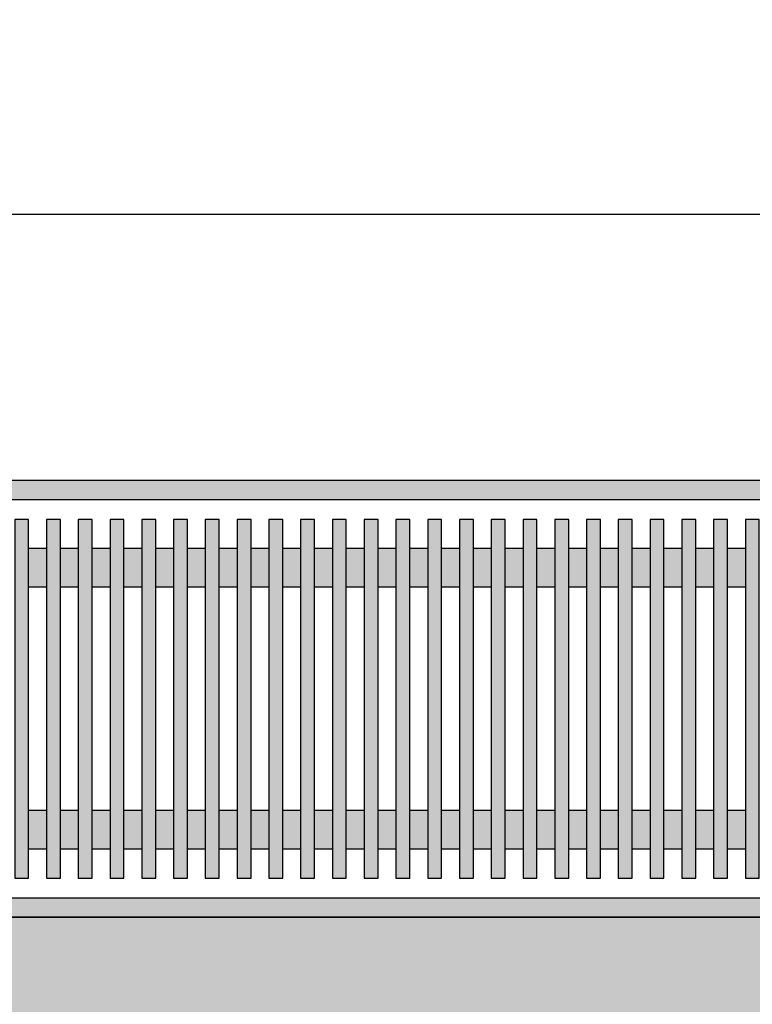
# Model space of a CAD drawing. Units: inches. Extents: x 3592 to 4861, y 1650 to 2243.
# Tile 13 of 30: x 4306 to 4335, y 1772 to 1812. Entities that reach past the tile are written whole.
import ezdxf

# ---------------------------------------------------------------- set-up
doc = ezdxf.new("R2010")
doc.units = ezdxf.units.IN
for name, color, linetype, lineweight in [('A-ANNO-DIMS', 2, 'Continuous', 13), ('A-FURN', 9, 'Continuous', 13), ('A-WALL', 7, 'Continuous', 35), ('estofado', 7, 'Continuous', 25)]:
    doc.layers.add(name, color=color, linetype=linetype, lineweight=lineweight)
doc.layers.add('A-WALL-PATT', color=252, linetype='Continuous', lineweight=13, true_color=0x939598)
doc.layers.add('MOBIL', color=7, linetype='Continuous')
doc.styles.get("Standard").update_dxf_attribs({"font": 'arial.ttf'})
doc.dimstyles.new('ISO-25', dxfattribs={"dimtxt": 9, "dimasz": 2.5, "dimexe": 1.25, "dimexo": 0.625, "dimtad": 1, "dimlunit": 3, "dimtxsty": 'Standard', "dimcen": 2.5, "dimadec": 0, "dimazin": 0, "dimtfac": 1, "dimtmove": 0, "dimatfit": 3, "dimfxl": 1, "dimarcsym": 0})

# ---------------------------------------------------------------- blocks, each defined once
blk = doc.blocks.new('Aparador Aido WV')
at = {"layer": 'MOBIL'}
h = blk.add_hatch(color=256, dxfattribs=at)
h.set_gradient(color1=(226, 228, 228), one_color=1, tint=1, name='CYLINDER')
h.paths.add_polyline_path([(0.9, -0.02), (0.9, 0), (-0.9, 0), (-0.9, -0.02)])
h = blk.add_hatch(color=256, dxfattribs=at)
h.set_gradient(color1=(106, 79, 62), color2=(55, 41, 32), one_color=1, tint=0.17)
h.paths.add_polyline_path([(-0.2072, -0.4098), (-0.1928, -0.4098), (-0.1928, -0.0402), (-0.2072, -0.0402)])
h = blk.add_hatch(color=256, dxfattribs=at)
h.set_gradient(color1=(106, 79, 62), color2=(55, 41, 32), one_color=1, tint=0.17)
h.paths.add_polyline_path([(-0.1744, -0.0402), (-0.1744, -0.4098), (-0.1601, -0.4098), (-0.1601, -0.0402)])
h = blk.add_hatch(color=256, dxfattribs=at)
h.set_gradient(color1=(106, 79, 62), color2=(55, 41, 32), one_color=1, tint=0.17)
h.paths.add_polyline_path([(-0.1417, -0.0402), (-0.1417, -0.4098), (-0.1273, -0.4098), (-0.1273, -0.0402)])
h = blk.add_hatch(color=256, dxfattribs=at)
h.set_gradient(color1=(106, 79, 62), color2=(55, 41, 32), one_color=1, tint=0.17)
h.paths.add_polyline_path([(-0.1089, -0.0402), (-0.1089, -0.4098), (-0.0946, -0.4098), (-0.0946, -0.0402)])
h = blk.add_hatch(color=256, dxfattribs=at)
h.set_gradient(color1=(106, 79, 62), color2=(55, 41, 32), one_color=1, tint=0.17)
h.paths.add_polyline_path([(-0.0762, -0.0402), (-0.0762, -0.4098), (-0.0618, -0.4098), (-0.0618, -0.0402)])
h = blk.add_hatch(color=256, dxfattribs=at)
h.set_gradient(color1=(106, 79, 62), color2=(55, 41, 32), one_color=1, tint=0.17)
h.paths.add_polyline_path([(-0.0434, -0.0402), (-0.0434, -0.4098), (-0.0291, -0.4098), (-0.0291, -0.0402)])
h = blk.add_hatch(color=256, dxfattribs=at)
h.set_gradient(color1=(106, 79, 62), color2=(55, 41, 32), one_color=1, tint=0.17)
h.paths.add_polyline_path([(-0.0107, -0.0402), (-0.0107, -0.4098), (0.0037, -0.4098), (0.0037, -0.0402)])
h = blk.add_hatch(color=256, dxfattribs=at)
h.set_gradient(color1=(106, 79, 62), color2=(55, 41, 32), one_color=1, tint=0.17)
h.paths.add_polyline_path([(0.0221, -0.0402), (0.0221, -0.4098), (0.0364, -0.4098), (0.0364, -0.0402)])
h = blk.add_hatch(color=256, dxfattribs=at)
h.set_gradient(color1=(106, 79, 62), color2=(55, 41, 32), one_color=1, tint=0.17)
h.paths.add_polyline_path([(0.0548, -0.0402), (0.0548, -0.4098), (0.0692, -0.4098), (0.0692, -0.0402)])
h = blk.add_hatch(color=256, dxfattribs=at)
h.set_gradient(color1=(106, 79, 62), color2=(55, 41, 32), one_color=1, tint=0.17)
h.paths.add_polyline_path([(0.1019, -0.0402), (0.0876, -0.0402), (0.0876, -0.4098), (0.1019, -0.4098)])
h = blk.add_hatch(color=256, dxfattribs=at)
h.set_gradient(color1=(106, 79, 62), color2=(55, 41, 32), one_color=1, tint=0.17)
h.paths.add_polyline_path([(0.1203, -0.0402), (0.1203, -0.4098), (0.1347, -0.4098), (0.1347, -0.0402)])
h = blk.add_hatch(color=256, dxfattribs=at)
h.set_gradient(color1=(106, 79, 62), color2=(55, 41, 32), one_color=1, tint=0.17)
h.paths.add_polyline_path([(0.1531, -0.0402), (0.1531, -0.4098), (0.1675, -0.4098), (0.1675, -0.0402)])
h = blk.add_hatch(color=256, dxfattribs=at)
h.set_gradient(color1=(106, 79, 62), color2=(55, 41, 32), one_color=1, tint=0.17)
h.paths.add_polyline_path([(0.1858, -0.0402), (0.1858, -0.4098), (0.2002, -0.4098), (0.2002, -0.0402)])
h = blk.add_hatch(color=256, dxfattribs=at)
h.set_gradient(color1=(106, 79, 62), color2=(55, 41, 32), one_color=1, tint=0.17)
h.paths.add_polyline_path([(0.2186, -0.0402), (0.2186, -0.4098), (0.233, -0.4098), (0.233, -0.0402)])
h = blk.add_hatch(color=256, dxfattribs=at)
h.set_gradient(color1=(106, 79, 62), color2=(55, 41, 32), one_color=1, tint=0.17)
h.paths.add_polyline_path([(0.2513, -0.0402), (0.2513, -0.4098), (0.2657, -0.4098), (0.2657, -0.0402)])
h = blk.add_hatch(color=256, dxfattribs=at)
h.set_gradient(color1=(106, 79, 62), color2=(55, 41, 32), one_color=1, tint=0.17)
h.paths.add_polyline_path([(0.2841, -0.0402), (0.2841, -0.4098), (0.2985, -0.4098), (0.2985, -0.0402)])
h = blk.add_hatch(color=256, dxfattribs=at)
h.set_gradient(color1=(106, 79, 62), color2=(55, 41, 32), one_color=1, tint=0.17)
h.paths.add_polyline_path([(0.3168, -0.0402), (0.3168, -0.4098), (0.3312, -0.4098), (0.3312, -0.0402)])
h = blk.add_hatch(color=256, dxfattribs=at)
h.set_gradient(color1=(106, 79, 62), color2=(55, 41, 32), one_color=1, tint=0.17)
h.paths.add_polyline_path([(0.3496, -0.0402), (0.3496, -0.4098), (0.364, -0.4098), (0.364, -0.0402)])
h = blk.add_hatch(color=256, dxfattribs=at)
h.set_gradient(color1=(106, 79, 62), color2=(55, 41, 32), one_color=1, tint=0.17)
h.paths.add_polyline_path([(0.3823, -0.0402), (0.3823, -0.4098), (0.3967, -0.4098), (0.3967, -0.0402)])
h = blk.add_hatch(color=256, dxfattribs=at)
h.set_gradient(color1=(106, 79, 62), color2=(55, 41, 32), one_color=1, tint=0.17)
h.paths.add_polyline_path([(0.4151, -0.4098), (0.4295, -0.4098), (0.4295, -0.0402), (0.4151, -0.0402)])
h = blk.add_hatch(color=256, dxfattribs=at)
h.set_gradient(color1=(106, 79, 62), color2=(55, 41, 32), one_color=1, tint=0.17)
h.paths.add_polyline_path([(0.4479, -0.0402), (0.4479, -0.4098), (0.4622, -0.4098), (0.4622, -0.0402)])
h = blk.add_hatch(color=256, dxfattribs=at)
h.set_gradient(color1=(106, 79, 62), color2=(55, 41, 32), one_color=1, tint=0.17)
h.paths.add_polyline_path([(0.4806, -0.0402), (0.4806, -0.4098), (0.495, -0.4098), (0.495, -0.0402)])
h = blk.add_hatch(color=256, dxfattribs=at)
h.set_gradient(color1=(106, 79, 62), color2=(55, 41, 32), one_color=1, tint=0.17)
h.paths.add_polyline_path([(0.5134, -0.0402), (0.5134, -0.4098), (0.5277, -0.4098), (0.5277, -0.0402)])
h = blk.add_hatch(color=256, dxfattribs=at)
h.set_gradient(color1=(106, 79, 62), color2=(55, 41, 32), one_color=1, tint=0.17)
h.paths.add_polyline_path([(0.5461, -0.0402), (0.5461, -0.4098), (0.5605, -0.4098), (0.5605, -0.0402)])
h = blk.add_hatch(color=256, dxfattribs=at)
h.set_gradient(color1=(106, 79, 62), color2=(157, 117, 92), one_color=1, tint=0.49)
h.paths.add_polyline_path([(-0.1744, -0.07), (-0.1928, -0.07), (-0.1928, -0.11), (-0.1744, -0.11)])
h = blk.add_hatch(color=256, dxfattribs=at)
h.set_gradient(color1=(106, 79, 62), color2=(157, 117, 92), one_color=1, tint=0.49)
h.paths.add_polyline_path([(-0.1417, -0.07), (-0.1601, -0.07), (-0.1601, -0.11), (-0.1417, -0.11)])
h = blk.add_hatch(color=256, dxfattribs=at)
h.set_gradient(color1=(106, 79, 62), color2=(157, 117, 92), one_color=1, tint=0.49)
h.paths.add_polyline_path([(-0.1089, -0.07), (-0.1273, -0.07), (-0.1273, -0.11), (-0.1089, -0.11)])
h = blk.add_hatch(color=256, dxfattribs=at)
h.set_gradient(color1=(106, 79, 62), color2=(157, 117, 92), one_color=1, tint=0.49)
h.paths.add_polyline_path([(-0.0762, -0.07), (-0.0946, -0.07), (-0.0946, -0.11), (-0.0762, -0.11)])
h = blk.add_hatch(color=256, dxfattribs=at)
h.set_gradient(color1=(106, 79, 62), color2=(157, 117, 92), one_color=1, tint=0.49)
h.paths.add_polyline_path([(-0.0434, -0.07), (-0.0618, -0.07), (-0.0618, -0.11), (-0.0434, -0.11)])
h = blk.add_hatch(color=256, dxfattribs=at)
h.set_gradient(color1=(106, 79, 62), color2=(157, 117, 92), one_color=1, tint=0.49)
h.paths.add_polyline_path([(-0.0107, -0.07), (-0.0291, -0.07), (-0.0291, -0.11), (-0.0107, -0.11)])
h = blk.add_hatch(color=256, dxfattribs=at)
h.set_gradient(color1=(106, 79, 62), color2=(157, 117, 92), one_color=1, tint=0.49)
h.paths.add_polyline_path([(0.0221, -0.07), (0.0037, -0.07), (0.0037, -0.11), (0.0221, -0.11)])
h = blk.add_hatch(color=256, dxfattribs=at)
h.set_gradient(color1=(106, 79, 62), color2=(157, 117, 92), one_color=1, tint=0.49)
h.paths.add_polyline_path([(0.0548, -0.07), (0.0364, -0.07), (0.0364, -0.11), (0.0548, -0.11)])
h = blk.add_hatch(color=256, dxfattribs=at)
h.set_gradient(color1=(106, 79, 62), color2=(157, 117, 92), one_color=1, tint=0.49)
h.paths.add_polyline_path([(0.0876, -0.07), (0.0692, -0.07), (0.0692, -0.11), (0.0876, -0.11)])
h = blk.add_hatch(color=256, dxfattribs=at)
h.set_gradient(color1=(106, 79, 62), color2=(157, 117, 92), one_color=1, tint=0.49)
h.paths.add_polyline_path([(0.1203, -0.07), (0.1019, -0.07), (0.1019, -0.11), (0.1203, -0.11)])
h = blk.add_hatch(color=256, dxfattribs=at)
h.set_gradient(color1=(106, 79, 62), color2=(157, 117, 92), one_color=1, tint=0.49)
h.paths.add_polyline_path([(0.1531, -0.07), (0.1347, -0.07), (0.1347, -0.11), (0.1531, -0.11)])
h = blk.add_hatch(color=256, dxfattribs=at)
h.set_gradient(color1=(106, 79, 62), color2=(157, 117, 92), one_color=1, tint=0.49)
h.paths.add_polyline_path([(0.1858, -0.07), (0.1675, -0.07), (0.1675, -0.11), (0.1858, -0.11)])
h = blk.add_hatch(color=256, dxfattribs=at)
h.set_gradient(color1=(106, 79, 62), color2=(157, 117, 92), one_color=1, tint=0.49)
h.paths.add_polyline_path([(0.2186, -0.07), (0.2002, -0.07), (0.2002, -0.11), (0.2186, -0.11)])
h = blk.add_hatch(color=256, dxfattribs=at)
h.set_gradient(color1=(106, 79, 62), color2=(157, 117, 92), one_color=1, tint=0.49)
h.paths.add_polyline_path([(0.2513, -0.07), (0.233, -0.07), (0.233, -0.11), (0.2513, -0.11)])
h = blk.add_hatch(color=256, dxfattribs=at)
h.set_gradient(color1=(106, 79, 62), color2=(157, 117, 92), one_color=1, tint=0.49)
h.paths.add_polyline_path([(0.2841, -0.07), (0.2657, -0.07), (0.2657, -0.11), (0.2841, -0.11)])
h = blk.add_hatch(color=256, dxfattribs=at)
h.set_gradient(color1=(106, 79, 62), color2=(157, 117, 92), one_color=1, tint=0.49)
h.paths.add_polyline_path([(0.3168, -0.07), (0.2985, -0.07), (0.2985, -0.11), (0.3168, -0.11)])
h = blk.add_hatch(color=256, dxfattribs=at)
h.set_gradient(color1=(106, 79, 62), color2=(157, 117, 92), one_color=1, tint=0.49)
h.paths.add_polyline_path([(0.3496, -0.07), (0.3312, -0.07), (0.3312, -0.11), (0.3496, -0.11)])
h = blk.add_hatch(color=256, dxfattribs=at)
h.set_gradient(color1=(106, 79, 62), color2=(157, 117, 92), one_color=1, tint=0.49)
h.paths.add_polyline_path([(0.3823, -0.07), (0.364, -0.07), (0.364, -0.11), (0.3823, -0.11)])
h = blk.add_hatch(color=256, dxfattribs=at)
h.set_gradient(color1=(106, 79, 62), color2=(157, 117, 92), one_color=1, tint=0.49)
h.paths.add_polyline_path([(0.4151, -0.07), (0.3967, -0.07), (0.3967, -0.11), (0.4151, -0.11)])
h = blk.add_hatch(color=256, dxfattribs=at)
h.set_gradient(color1=(106, 79, 62), color2=(157, 117, 92), one_color=1, tint=0.49)
h.paths.add_polyline_path([(0.4479, -0.07), (0.4295, -0.07), (0.4295, -0.11), (0.4479, -0.11)])
h = blk.add_hatch(color=256, dxfattribs=at)
h.set_gradient(color1=(106, 79, 62), color2=(157, 117, 92), one_color=1, tint=0.49)
h.paths.add_polyline_path([(0.4806, -0.07), (0.4622, -0.07), (0.4622, -0.11), (0.4806, -0.11)])
h = blk.add_hatch(color=256, dxfattribs=at)
h.set_gradient(color1=(106, 79, 62), color2=(157, 117, 92), one_color=1, tint=0.49)
h.paths.add_polyline_path([(0.5134, -0.07), (0.495, -0.07), (0.495, -0.11), (0.5134, -0.11)])
h = blk.add_hatch(color=256, dxfattribs=at)
h.set_gradient(color1=(106, 79, 62), color2=(157, 117, 92), one_color=1, tint=0.49)
h.paths.add_polyline_path([(0.5277, -0.11), (0.5461, -0.11), (0.5461, -0.07), (0.5277, -0.07)])
h = blk.add_hatch(color=256, dxfattribs=at)
h.set_gradient(color1=(106, 79, 62), color2=(157, 117, 92), one_color=1, tint=0.49)
h.paths.add_polyline_path([(-0.1744, -0.34), (-0.1928, -0.34), (-0.1928, -0.38), (-0.1744, -0.38)])
h = blk.add_hatch(color=256, dxfattribs=at)
h.set_gradient(color1=(106, 79, 62), color2=(157, 117, 92), one_color=1, tint=0.49)
h.paths.add_polyline_path([(-0.1417, -0.34), (-0.1601, -0.34), (-0.1601, -0.38), (-0.1417, -0.38)])
h = blk.add_hatch(color=256, dxfattribs=at)
h.set_gradient(color1=(106, 79, 62), color2=(157, 117, 92), one_color=1, tint=0.49)
h.paths.add_polyline_path([(-0.1089, -0.34), (-0.1273, -0.34), (-0.1273, -0.38), (-0.1089, -0.38)])
h = blk.add_hatch(color=256, dxfattribs=at)
h.set_gradient(color1=(106, 79, 62), color2=(157, 117, 92), one_color=1, tint=0.49)
h.paths.add_polyline_path([(-0.0762, -0.34), (-0.0946, -0.34), (-0.0946, -0.38), (-0.0762, -0.38)])
h = blk.add_hatch(color=256, dxfattribs=at)
h.set_gradient(color1=(106, 79, 62), color2=(157, 117, 92), one_color=1, tint=0.49)
h.paths.add_polyline_path([(-0.0434, -0.34), (-0.0618, -0.34), (-0.0618, -0.38), (-0.0434, -0.38)])
h = blk.add_hatch(color=256, dxfattribs=at)
h.set_gradient(color1=(106, 79, 62), color2=(157, 117, 92), one_color=1, tint=0.49)
h.paths.add_polyline_path([(-0.0107, -0.34), (-0.0291, -0.34), (-0.0291, -0.38), (-0.0107, -0.38)])
h = blk.add_hatch(color=256, dxfattribs=at)
h.set_gradient(color1=(106, 79, 62), color2=(157, 117, 92), one_color=1, tint=0.49)
h.paths.add_polyline_path([(0.0221, -0.34), (0.0037, -0.34), (0.0037, -0.38), (0.0221, -0.38)])
h = blk.add_hatch(color=256, dxfattribs=at)
h.set_gradient(color1=(106, 79, 62), color2=(157, 117, 92), one_color=1, tint=0.49)
h.paths.add_polyline_path([(0.0548, -0.34), (0.0364, -0.34), (0.0364, -0.38), (0.0548, -0.38)])
h = blk.add_hatch(color=256, dxfattribs=at)
h.set_gradient(color1=(106, 79, 62), color2=(157, 117, 92), one_color=1, tint=0.49)
h.paths.add_polyline_path([(0.0876, -0.34), (0.0692, -0.34), (0.0692, -0.38), (0.0876, -0.38)])
h = blk.add_hatch(color=256, dxfattribs=at)
h.set_gradient(color1=(106, 79, 62), color2=(157, 117, 92), one_color=1, tint=0.49)
h.paths.add_polyline_path([(0.1203, -0.34), (0.1019, -0.34), (0.1019, -0.38), (0.1203, -0.38)])
h = blk.add_hatch(color=256, dxfattribs=at)
h.set_gradient(color1=(106, 79, 62), color2=(157, 117, 92), one_color=1, tint=0.49)
h.paths.add_polyline_path([(0.1531, -0.34), (0.1347, -0.34), (0.1347, -0.38), (0.1531, -0.38)])
h = blk.add_hatch(color=256, dxfattribs=at)
h.set_gradient(color1=(106, 79, 62), color2=(157, 117, 92), one_color=1, tint=0.49)
h.paths.add_polyline_path([(0.1858, -0.34), (0.1675, -0.34), (0.1675, -0.38), (0.1858, -0.38)])
h = blk.add_hatch(color=256, dxfattribs=at)
h.set_gradient(color1=(106, 79, 62), color2=(157, 117, 92), one_color=1, tint=0.49)
h.paths.add_polyline_path([(0.2186, -0.34), (0.2002, -0.34), (0.2002, -0.38), (0.2186, -0.38)])
h = blk.add_hatch(color=256, dxfattribs=at)
h.set_gradient(color1=(106, 79, 62), color2=(157, 117, 92), one_color=1, tint=0.49)
h.paths.add_polyline_path([(0.2513, -0.34), (0.233, -0.34), (0.233, -0.38), (0.2513, -0.38)])
h = blk.add_hatch(color=256, dxfattribs=at)
h.set_gradient(color1=(106, 79, 62), color2=(157, 117, 92), one_color=1, tint=0.49)
h.paths.add_polyline_path([(0.2841, -0.34), (0.2657, -0.34), (0.2657, -0.38), (0.2841, -0.38)])
h = blk.add_hatch(color=256, dxfattribs=at)
h.set_gradient(color1=(106, 79, 62), color2=(157, 117, 92), one_color=1, tint=0.49)
h.paths.add_polyline_path([(0.3168, -0.34), (0.2985, -0.34), (0.2985, -0.38), (0.3168, -0.38)])
h = blk.add_hatch(color=256, dxfattribs=at)
h.set_gradient(color1=(106, 79, 62), color2=(157, 117, 92), one_color=1, tint=0.49)
h.paths.add_polyline_path([(0.3496, -0.34), (0.3312, -0.34), (0.3312, -0.38), (0.3496, -0.38)])
h = blk.add_hatch(color=256, dxfattribs=at)
h.set_gradient(color1=(106, 79, 62), color2=(157, 117, 92), one_color=1, tint=0.49)
h.paths.add_polyline_path([(0.3823, -0.34), (0.364, -0.34), (0.364, -0.38), (0.3823, -0.38)])
h = blk.add_hatch(color=256, dxfattribs=at)
h.set_gradient(color1=(106, 79, 62), color2=(157, 117, 92), one_color=1, tint=0.49)
h.paths.add_polyline_path([(0.4151, -0.34), (0.3967, -0.34), (0.3967, -0.38), (0.4151, -0.38)])
h = blk.add_hatch(color=256, dxfattribs=at)
h.set_gradient(color1=(106, 79, 62), color2=(157, 117, 92), one_color=1, tint=0.49)
h.paths.add_polyline_path([(0.4479, -0.34), (0.4295, -0.34), (0.4295, -0.38), (0.4479, -0.38)])
h = blk.add_hatch(color=256, dxfattribs=at)
h.set_gradient(color1=(106, 79, 62), color2=(157, 117, 92), one_color=1, tint=0.49)
h.paths.add_polyline_path([(0.4806, -0.34), (0.4622, -0.34), (0.4622, -0.38), (0.4806, -0.38)])
h = blk.add_hatch(color=256, dxfattribs=at)
h.set_gradient(color1=(106, 79, 62), color2=(157, 117, 92), one_color=1, tint=0.49)
h.paths.add_polyline_path([(0.5134, -0.34), (0.495, -0.34), (0.495, -0.38), (0.5134, -0.38)])
h = blk.add_hatch(color=256, dxfattribs=at)
h.set_gradient(color1=(106, 79, 62), color2=(157, 117, 92), one_color=1, tint=0.49)
h.paths.add_polyline_path([(0.5461, -0.34), (0.5277, -0.34), (0.5277, -0.38), (0.5461, -0.38)])
h = blk.add_hatch(color=256, dxfattribs=at)
h.set_gradient(color1=(226, 228, 228), one_color=1, tint=1, name='CYLINDER')
h.paths.add_polyline_path([(0.9, -0.45), (0.9, -0.43), (-0.9, -0.43), (-0.9, -0.45)])
at = {"layer": 'estofado', "ltscale": 0.5}
for p, q in [((-0.1928, -0.07), (-0.1744, -0.07)), ((-0.1601, -0.07), (-0.1417, -0.07)), ((-0.1273, -0.07), (-0.1089, -0.07)), ((-0.0946, -0.07), (-0.0762, -0.07)), ((-0.0618, -0.07), (-0.0434, -0.07)), ((-0.0291, -0.07), (-0.0107, -0.07)), ((0.0037, -0.07), (0.0221, -0.07)), ((0.0364, -0.07), (0.0548, -0.07)), ((0.0692, -0.07), (0.0876, -0.07)), ((0.1019, -0.07), (0.1203, -0.07)), ((0.1347, -0.07), (0.1531, -0.07)), ((0.1675, -0.07), (0.1858, -0.07)), ((0.2002, -0.07), (0.2186, -0.07)), ((0.233, -0.07), (0.2513, -0.07)), ((0.2657, -0.07), (0.2841, -0.07)), ((0.2985, -0.07), (0.3168, -0.07)), ((0.3312, -0.07), (0.3496, -0.07)), ((0.364, -0.07), (0.3823, -0.07)), ((0.3967, -0.07), (0.4151, -0.07)), ((0.4295, -0.07), (0.4479, -0.07)), ((0.4622, -0.07), (0.4806, -0.07)), ((0.495, -0.07), (0.5134, -0.07)), ((0.5277, -0.07), (0.5461, -0.07)), ((-0.1928, -0.11), (-0.1744, -0.11)), ((-0.1601, -0.11), (-0.1417, -0.11)), ((-0.1273, -0.11), (-0.1089, -0.11)), ((-0.0946, -0.11), (-0.0762, -0.11)), ((-0.0618, -0.11), (-0.0434, -0.11)), ((-0.0291, -0.11), (-0.0107, -0.11)), ((0.0037, -0.11), (0.0221, -0.11)), ((0.0364, -0.11), (0.0548, -0.11)), ((0.0692, -0.11), (0.0876, -0.11)), ((0.1019, -0.11), (0.1203, -0.11)), ((0.1347, -0.11), (0.1531, -0.11)), ((0.1675, -0.11), (0.1858, -0.11)), ((0.2002, -0.11), (0.2186, -0.11)), ((0.233, -0.11), (0.2513, -0.11)), ((0.2657, -0.11), (0.2841, -0.11)), ((0.2985, -0.11), (0.3168, -0.11)), ((0.3312, -0.11), (0.3496, -0.11)), ((0.364, -0.11), (0.3823, -0.11)), ((0.3967, -0.11), (0.4151, -0.11)), ((0.4295, -0.11), (0.4479, -0.11)), ((0.4622, -0.11), (0.4806, -0.11)), ((0.495, -0.11), (0.5134, -0.11)), ((0.5277, -0.11), (0.5461, -0.11)), ((-0.1928, -0.34), (-0.1744, -0.34)), ((-0.1601, -0.34), (-0.1417, -0.34)), ((-0.1273, -0.34), (-0.1089, -0.34)), ((-0.0946, -0.34), (-0.0762, -0.34)), ((-0.0618, -0.34), (-0.0434, -0.34)), ((-0.0291, -0.34), (-0.0107, -0.34)), ((0.0037, -0.34), (0.0221, -0.34)), ((0.0364, -0.34), (0.0548, -0.34)), ((0.0692, -0.34), (0.0876, -0.34)), ((0.1019, -0.34), (0.1203, -0.34)), ((0.1347, -0.34), (0.1531, -0.34)), ((0.1675, -0.34), (0.1858, -0.34)), ((0.2002, -0.34), (0.2186, -0.34)), ((0.233, -0.34), (0.2513, -0.34)), ((0.2657, -0.34), (0.2841, -0.34)), ((0.2985, -0.34), (0.3168, -0.34)), ((0.3312, -0.34), (0.3496, -0.34)), ((0.364, -0.34), (0.3823, -0.34)), ((0.3967, -0.34), (0.4151, -0.34)), ((0.4295, -0.34), (0.4479, -0.34)), ((0.4622, -0.34), (0.4806, -0.34)), ((0.495, -0.34), (0.5134, -0.34)), ((0.5277, -0.34), (0.5461, -0.34)), ((-0.1928, -0.38), (-0.1744, -0.38)), ((-0.1601, -0.38), (-0.1417, -0.38)), ((-0.1273, -0.38), (-0.1089, -0.38)), ((-0.0946, -0.38), (-0.0762, -0.38)), ((-0.0618, -0.38), (-0.0434, -0.38)), ((-0.0291, -0.38), (-0.0107, -0.38)), ((0.0037, -0.38), (0.0221, -0.38)), ((0.0364, -0.38), (0.0548, -0.38)), ((0.0692, -0.38), (0.0876, -0.38)), ((0.1019, -0.38), (0.1203, -0.38)), ((0.1347, -0.38), (0.1531, -0.38)), ((0.1675, -0.38), (0.1858, -0.38)), ((0.2002, -0.38), (0.2186, -0.38)), ((0.233, -0.38), (0.2513, -0.38)), ((0.2657, -0.38), (0.2841, -0.38)), ((0.2985, -0.38), (0.3168, -0.38)), ((0.3312, -0.38), (0.3496, -0.38)), ((0.364, -0.38), (0.3823, -0.38)), ((0.3967, -0.38), (0.4151, -0.38)), ((0.4295, -0.38), (0.4479, -0.38)), ((0.4622, -0.38), (0.4806, -0.38)), ((0.495, -0.38), (0.5134, -0.38)), ((0.5277, -0.38), (0.5461, -0.38))]:
    blk.add_line(p, q, dxfattribs=at)
for points in [[(-0.2072, -0.0402), (-0.2072, -0.4098), (-0.1928, -0.4098), (-0.1928, -0.0402)], [(-0.1744, -0.0402), (-0.1744, -0.4098), (-0.1601, -0.4098), (-0.1601, -0.0402)], [(-0.1417, -0.0402), (-0.1417, -0.4098), (-0.1273, -0.4098), (-0.1273, -0.0402)], [(-0.1089, -0.0402), (-0.1089, -0.4098), (-0.0946, -0.4098), (-0.0946, -0.0402)], [(-0.0762, -0.0402), (-0.0762, -0.4098), (-0.0618, -0.4098), (-0.0618, -0.0402)], [(-0.0434, -0.0402), (-0.0434, -0.4098), (-0.0291, -0.4098), (-0.0291, -0.0402)], [(-0.0107, -0.0402), (-0.0107, -0.4098), (0.0037, -0.4098), (0.0037, -0.0402)], [(0.0221, -0.0402), (0.0221, -0.4098), (0.0364, -0.4098), (0.0364, -0.0402)], [(0.0548, -0.0402), (0.0548, -0.4098), (0.0692, -0.4098), (0.0692, -0.0402)], [(0.0876, -0.0402), (0.0876, -0.4098), (0.1019, -0.4098), (0.1019, -0.0402)], [(0.1203, -0.0402), (0.1203, -0.4098), (0.1347, -0.4098), (0.1347, -0.0402)], [(0.1531, -0.0402), (0.1531, -0.4098), (0.1675, -0.4098), (0.1675, -0.0402)], [(0.1858, -0.0402), (0.1858, -0.4098), (0.2002, -0.4098), (0.2002, -0.0402)], [(0.2186, -0.0402), (0.2186, -0.4098), (0.233, -0.4098), (0.233, -0.0402)], [(0.2513, -0.0402), (0.2513, -0.4098), (0.2657, -0.4098), (0.2657, -0.0402)], [(0.2841, -0.0402), (0.2841, -0.4098), (0.2985, -0.4098), (0.2985, -0.0402)], [(0.3168, -0.0402), (0.3168, -0.4098), (0.3312, -0.4098), (0.3312, -0.0402)], [(0.3496, -0.0402), (0.3496, -0.4098), (0.364, -0.4098), (0.364, -0.0402)], [(0.3823, -0.0402), (0.3823, -0.4098), (0.3967, -0.4098), (0.3967, -0.0402)], [(0.4151, -0.0402), (0.4151, -0.4098), (0.4295, -0.4098), (0.4295, -0.0402)], [(0.4479, -0.0402), (0.4479, -0.4098), (0.4622, -0.4098), (0.4622, -0.0402)], [(0.4806, -0.0402), (0.4806, -0.4098), (0.495, -0.4098), (0.495, -0.0402)], [(0.5134, -0.0402), (0.5134, -0.4098), (0.5277, -0.4098), (0.5277, -0.0402)], [(0.5461, -0.0402), (0.5461, -0.4098), (0.5605, -0.4098), (0.5605, -0.0402)]]:
    blk.add_lwpolyline(points, close=True, dxfattribs=at)
at = {"layer": 'MOBIL'}
for p, q in [((0.9, -0.02), (-0.9, -0.02)), ((-0.9, -0.43), (0.9, -0.43))]:
    blk.add_line(p, q, dxfattribs=at)
blk.add_lwpolyline([(-0.9, -0.45), (0.9, -0.45), (0.9, 0), (-0.9, 0)], close=True, dxfattribs=at)
blk = doc.blocks.new('*D156')
at = {"layer": 'A-ANNO-DIMS', "color": 0, "lineweight": -2, "transparency": 16777216}
for p, q in [((4291.393, 1793.561), (4291.393, 1804.979)), ((4363.347, 1793.561), (4363.347, 1804.979)), ((4291.393, 1803.729), (4155.277, 1803.729)), ((4360.847, 1803.729), (4293.893, 1803.729))]:
    blk.add_line(p, q, dxfattribs=at)
at = {"layer": 'A-ANNO-DIMS', "color": 0, "transparency": 16777216}
for points in [[(4293.893, 1804.145), (4293.893, 1803.312), (4291.393, 1803.729)], [(4360.847, 1804.145), (4360.847, 1803.312), (4363.347, 1803.729)]]:
    blk.add_solid(points, dxfattribs=at)
at = {"layer": 'Defpoints', "color": 0, "transparency": 16777216}
for p in [(4291.393, 1803.729), (4291.393, 1792.936), (4363.347, 1792.936)]:
    blk.add_point(p, dxfattribs=at)
at = {"layer": 'A-ANNO-DIMS', "color": 0, "transparency": 16777216, "insert": (4222.085, 1809.01), "char_height": 9, "attachment_point": 5}
blk.add_mtext('SIDEBOARD 6\'-0" TYP.', dxfattribs=at)

msp = doc.modelspace()

# ---------------------------------------------------------------- hatches: boundary and pattern name
at = {"layer": 'A-WALL-PATT'}
h = msp.add_hatch(color=256, dxfattribs=at)
h.dxf.hatch_style = 1
h.paths.add_polyline_path([(4398.37, 2165.219), (4038.37, 2165.219), (4038.37, 1993.219), (4047.37, 1993.219), (4047.37, 2156.219), (4191.37, 2156.219), (4191.37, 2150.219), (4195.37, 2150.219), (4195.37, 2156.219), (4256.37, 2156.219), (4256.37, 2150.219), (4265.37, 2150.219), (4265.37, 2156.219), (4389.37, 2156.219), (4389.37, 2114.219), (4398.37, 2114.219)])
h.paths.add_polyline_path([(4265.37, 2102.219), (4256.37, 2102.219), (4256.37, 2096.219), (4195.37, 2096.219), (4195.37, 2102.219), (4191.37, 2102.219), (4191.37, 2020.219), (4195.37, 2020.219), (4195.37, 2087.219), (4256.37, 2087.219), (4256.37, 2020.219), (4306.37, 2020.219), (4306.37, 2024.219), (4265.37, 2024.219)], flags=17)
h.paths.add_polyline_path([(4398.37, 2066.219), (4389.37, 2066.219), (4389.37, 2024.219), (4348.37, 2024.219), (4348.37, 2020.219), (4389.37, 2020.219), (4389.37, 1989.719), (4398.37, 1989.719)])
h.paths.add_polyline_path([(4398.37, 1941.719), (4389.37, 1941.719), (4389.37, 1911.219), (4301.37, 1911.219), (4301.37, 1907.219), (4389.37, 1907.219), (4389.37, 1865.219), (4398.37, 1865.219)])
h.paths.add_polyline_path([(4398.37, 1817.219), (4389.37, 1817.219), (4389.37, 1775.219), (4265.37, 1775.219), (4265.37, 1911.219), (4256.37, 1911.219), (4256.37, 1817.219), (4220.87, 1817.219), (4220.87, 1808.219), (4256.37, 1808.219), (4256.37, 1766.219), (4389.37, 1766.219), (4389.37, 1694.219), (4256.37, 1694.219), (4256.37, 1685.219), (4398.37, 1685.219)])
h.paths.add_polyline_path([(4178.87, 1817.219), (4077.37, 1817.219), (4077.37, 1808.219), (4178.87, 1808.219)])
h.paths.add_polyline_path([(4111.37, 2020.219), (4155.37, 2020.219), (4155.37, 2024.219), (4077.37, 2024.219), (4077.37, 2020.219), (4107.37, 2020.219), (4107.37, 1942.219), (4047.37, 1942.219), (4047.37, 1969.219), (4038.37, 1969.219), (4038.37, 1911.219), (4047.37, 1911.219), (4047.37, 1938.219), (4107.37, 1938.219), (4107.37, 1860.219), (4077.37, 1860.219), (4077.37, 1856.219), (4111.37, 1856.219)])
h.paths.add_polyline_path([(4047.37, 1887.219), (4038.37, 1887.219), (4038.37, 1685.219), (4152.37, 1685.219), (4152.37, 1715.219), (4143.37, 1715.219), (4143.37, 1694.219), (4047.37, 1694.219)])
h.paths.add_polyline_path([(4152.37, 1772.219), (4143.37, 1772.219), (4143.37, 1751.219), (4152.37, 1751.219)], flags=17)

# ---------------------------------------------------------------- linework, layer by layer
at = {"layer": 'A-WALL'}
msp.add_line((4389.37, 1775.219), (4265.37, 1775.219), dxfattribs=at)

# ---------------------------------------------------------------- block references
at = {"layer": 'A-FURN', "xscale": 39.3701, "yscale": 39.3701, "zscale": 39.3701, "rotation": 180}
msp.add_blockref('Aparador Aido WV', (4327.37, 1775.219), dxfattribs=at)

# ---------------------------------------------------------------- dimensions: what is measured, and where the dimension line sits
at = {"layer": 'A-ANNO-DIMS'}
dim = msp.add_linear_dim(base=(4291.393, 1803.729), p1=(4363.347, 1792.936), p2=(4291.393, 1792.936), angle=180, text='SIDEBOARD <> TYP.', dimstyle='ISO-25', override={"dimdec": 1, "dimlfac": 1, "dimrnd": 0, "dimzin": 1, "dimdsep": 46, "dimlunit": 4, "dimfrac": 2}, dxfattribs=at)
dim.commit()
dim.dimension.update_dxf_attribs({"geometry": '*D156', "text_midpoint": (4222.085, 1809.01)})

doc.saveas('drawing.dxf')
